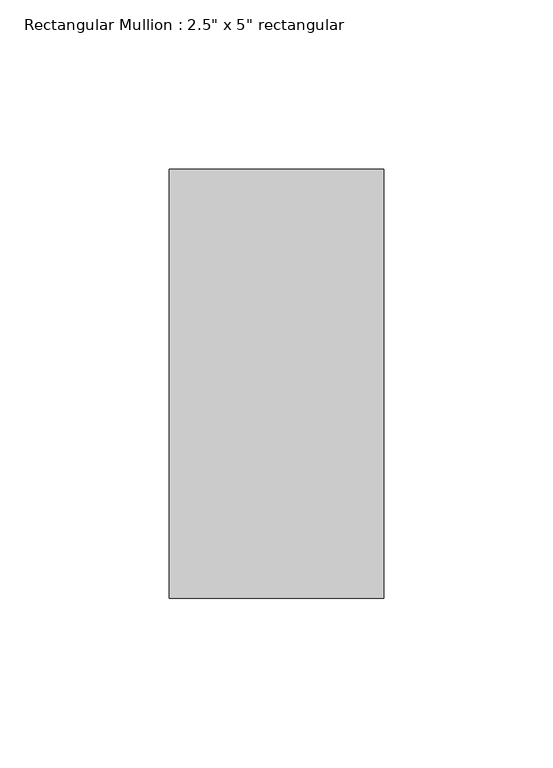
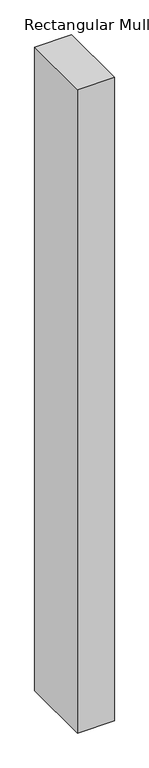
"""IFC4 building model written with IfcOpenShell, lengths in millimetres: member geometry."""

from ifc_helpers import new_model, si_unit, frame, origin, place, context, project, spatial, polyline, outline, extrude, source, transform, mapped, element, save


def member_b860638c(model_context):
    return source(origin(), model_context, "Body", "SweptSolid", [
        extrude(outline(polyline([(31.75, 63.5), (31.75, -63.5), (-31.75, -63.5), (-31.75, 63.5), (31.75, 63.5)])), frame((0.0, 0.0, -1168.8884615), z_axis=(0.0, 0.0, 1.0), x_axis=(1.0, 0.0, 0.0)), (0.0, 0.0, 1.0), 1168.8884615),
    ])


if __name__ == "__main__":
    model = new_model("IFC4")
    model_context = context("Model", 3, world=origin())
    ifc_project = project(units=[si_unit("LENGTHUNIT", "METRE", prefix="MILLI")], contexts=[model_context])
    site = spatial("IfcSite", under=ifc_project)
    building = spatial("IfcBuilding", under=site)
    placement = place(None, origin())
    member_shape = member_b860638c(model_context)
    element("IfcMember", 1, ObjectType="Rectangular Mullion : 2.5\" x 5\" rectangular", at=placement, inside=building, context=model_context, shape_type="MappedRepresentation", body=[
        mapped(member_shape, transform((0.0, 0.0, 0.0), x_axis=(1.0, 0.0, 0.0), y_axis=(0.0, 1.0, 0.0), z_axis=(0.0, 0.0, 1.0))),
    ])
    save(model, "model.ifc")

# Revit data of these elements
# Type "Rectangular Mullion : 2.5\" x 5\" rectangular"
#   built-in parameter 1007304 = 0.416667 (stored number, unit not read)
#   built-in parameter 1007301 = 0.104167 (stored number, unit not read)
#   built-in parameter 1007300 = 0.104167 (stored number, unit not read)
# Element 1 (IfcMember, "Rectangular Mullion : 2.5\" x 5\" rectangular")
#   Materials on its faces: "Aluminum"
# Materials
#   "Aluminum": class "Metal", colour RGB 247 247 247, transparency 0, Description = "Aluminum 6061", Cost = 0
